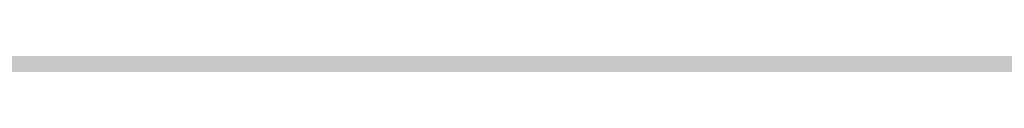
# Model space of a CAD drawing. Units: inches. Extents: x 2091 to 2899, y 967 to 2217.
# Tile 224 of 256: x 2203.4104 to 2203.7172, y 1152.2475 to 1152.2479. Entities that reach past the tile are written whole.
import ezdxf

# ---------------------------------------------------------------- set-up
doc = ezdxf.new("R2010")
doc.units = ezdxf.units.IN
doc.layers.add('A-WALL-PATT', color=141, linetype='Continuous', lineweight=13, true_color=0xadddf7)

msp = doc.modelspace()

# ---------------------------------------------------------------- hatches: boundary and pattern name
at = {"layer": 'A-WALL-PATT'}
h = msp.add_hatch(color=256, dxfattribs=at)
h.dxf.hatch_style = 1
h.paths.add_polyline_path([(2803.1436, 2050.91906), (2203.1436, 2050.91906), (2203.1436, 1090.91906), (2803.1436, 1090.91906)])
h.paths.add_polyline_path([(2635.79885, 1147.54046), (2674.52405, 1147.54046, 0.376086), (2678.52967, 1152.8802), (2678.52967, 1159.55647, 0.333335), (2674.52432, 1163.56185), (2674.52432, 1163.56185), (2674.52432, 1192.93439), (2635.80597, 1192.93439), (2597.08762, 1192.93439), (2597.08762, 1163.56185, 0.333335), (2593.08228, 1159.55647), (2593.08228, 1152.8802, 0.376086), (2597.08789, 1147.54046)], flags=0)
h.paths.add_polyline_path([(2436.01043, 1278.24078, 0.000483), (2435.95264, 1278.21503, -0.001328), (2435.93563, 1278.11169, -0.001711), (2436.11644, 1278.04076, 0.002185)], flags=0)
h.paths.add_polyline_path([(2794.1436, 1143.41906), (2794.1436, 1347.41906), (2543.37017, 1347.41906), (2543.37017, 1351.91906), (2794.1436, 1351.91906), (2794.1436, 1392.71355), (2793.9474, 1392.71355), (2793.9474, 1473.5369), (2794.1436, 1473.5369), (2794.1436, 1531.91906), (2650.1436, 1531.91906), (2650.1436, 1536.41906), (2794.1436, 1536.41906), (2794.1436, 1692.41906), (2609.37561, 1692.41906), (2609.37561, 1644.41906), (2604.87561, 1644.41906), (2604.87561, 1744.91906), (2609.37561, 1744.91906), (2609.37561, 1696.91906), (2794.1436, 1696.91906), (2794.1436, 1780.91906), (2609.6436, 1780.91906), (2493.87561, 1780.91906), (2493.87561, 1785.41906), (2609.6436, 1785.41906), (2794.1436, 1785.41906), (2794.1436, 1847.93882), (2793.95122, 1847.93882), (2793.95122, 1928.76217), (2794.1436, 1928.76217), (2794.1436, 1941.41906), (2614.1436, 1941.41906), (2614.1436, 1821.41906), (2609.6436, 1821.41906), (2609.6436, 1941.41906), (2392.1436, 1941.41906), (2392.1436, 1819.91906), (2387.6436, 1819.91906), (2387.6436, 1941.41906), (2212.1436, 1941.41906), (2212.1436, 1783.91906), (2392.1436, 1783.91906), (2392.1436, 1780.91906), (2212.1436, 1780.91906), (2212.1436, 1629.41906), (2387.6436, 1629.41906), (2387.6436, 1744.91906), (2392.1436, 1744.91906), (2392.1436, 1627.91906), (2317.1436, 1627.91906), (2317.1436, 1551.41906), (2317.1436, 1536.41906), (2459.38359, 1536.41906), (2459.38359, 1602.39648), (2463.88359, 1602.39648), (2463.88359, 1531.91906), (2456.6436, 1531.91906), (2456.6436, 1529.91906), (2452.1436, 1529.91906), (2452.1436, 1531.91906), (2312.6436, 1531.91906), (2312.6436, 1551.41906), (2306.1436, 1551.41906), (2306.1436, 1555.91906), (2308.1436, 1555.91906), (2308.1436, 1551.41906), (2312.6436, 1551.41906), (2312.6436, 1627.91906), (2212.1436, 1627.91906), (2212.1436, 1555.91906), (2270.1436, 1555.91906), (2270.1436, 1551.41906), (2212.1436, 1551.41906), (2212.1436, 1351.91906), (2272.1436, 1351.91906), (2272.1436, 1347.41906), (2212.1436, 1347.41906), (2212.1436, 1275.41906), (2308.1436, 1275.41906), (2308.1436, 1351.91906), (2452.1436, 1351.91906), (2452.1436, 1493.91906), (2456.6436, 1493.91906), (2456.6436, 1347.41906), (2312.6436, 1347.41906), (2312.6436, 1270.91906), (2212.1436, 1270.91906), (2212.1436, 1099.91906), (2281.23752, 1099.91906), (2282.87104, 1110.9138), (2282.00834, 1116.9966), (2278.55774, 1121.4204), (2268.20564, 1128.0562), (2272.08764, 1128.0562), (2273.81294, 1131.927), (2279.42034, 1134.6919), (2285.02784, 1135.2449), (2287.61584, 1137.4568), (2288.04714, 1138.0098), (2289.34114, 1140.7747), (2291.06654, 1139.6687), (2292.36054, 1135.2449), (2295.37984, 1136.9038), (2296.24254, 1135.7979), (2297.10524, 1133.033), (2300.12464, 1138.0098), (2303.14394, 1138.0098), (2304.43794, 1135.7979), (2303.14394, 1133.586), (2306.59464, 1134.6919), (2307.88874, 1133.033), (2310.90804, 1135.2449), (2313.92744, 1134.1389), (2315.62686, 1132.4271), (2308.32004, 1117.5496), (2290.20384, 1109.8079), (2288.90984, 1103.1721), (2289.27231, 1099.91906), (2434.91823, 1099.91906), (2431.59323, 1124.78806), (2429.93023, 1169.55306), (2430.92718, 1240.51969), (2435.65893, 1238.18613), (2437.13523, 1196.55406), (2438.79823, 1143.97306), (2442.67823, 1111.99806), (2446.55823, 1099.91906), (2794.1436, 1099.91906), (2794.1436, 1138.91906), (2548.03245, 1138.91906), (2548.03245, 1143.41906), (2548.03245, 1148.81906), (2546.66846, 1148.03156), (2528.68569, 1179.17862, 0.256256), (2512.03245, 1148.81906), (2512.03245, 1143.41906), (2512.03245, 1138.91906), (2507.53245, 1138.91906), (2507.53245, 1143.41906), (2507.53245, 1148.81906, 0.256256), (2490.8792, 1179.17862), (2472.89644, 1148.03156), (2471.53245, 1148.81906), (2471.53245, 1143.41906), (2467.03245, 1143.41906), (2467.03245, 1269.94579, 0.039061), (2460.90999, 1273.58006), (2467.03245, 1273.58006), (2467.03245, 1286.32536, 0.014511), (2465.21619, 1286.76191), (2467.03245, 1287.05258), (2467.03245, 1323.41906), (2471.53245, 1323.41906), (2471.53245, 1148.81906), (2489.53245, 1179.99597), (2490.89644, 1179.20847), (2490.8792, 1179.17862, -0.256256), (2507.53245, 1148.81906), (2507.53245, 1143.41906), (2512.03245, 1143.41906), (2512.03245, 1148.81906, -0.256256), (2528.68569, 1179.17862), (2528.66846, 1179.20847), (2530.03245, 1179.99597), (2548.03245, 1148.81906), (2548.03245, 1143.41906)], flags=16)
h.paths.add_polyline_path([(2607.76855, 1200.94508), (2607.76855, 1265.03063), (2597.08762, 1281.05201), (2619.78459, 1281.05201), (2627.79528, 1337.12686), (2635.79885, 1337.12686), (2643.81666, 1337.12686), (2651.82736, 1281.05201), (2674.52432, 1281.05201), (2663.8434, 1265.03063), (2663.8434, 1200.94508), (2635.80597, 1200.94508)], flags=0)
edge = h.paths.add_edge_path(flags=0)
edge.add_ellipse((13303.89622, 1272.99872), major_axis=(-10595.31304, 0), ratio=0.84230387009, start_angle=0.628237219, end_angle=0.6465541, ccw=False)
edge.add_ellipse((2711.70045, 1156.85268), major_axis=(2.21977, 0), ratio=0.8423039, start_angle=111.53524, end_angle=180.62824, ccw=False)
edge.add_ellipse((13303.15629, 1272.99872), major_axis=(-10593.02631, 0), ratio=0.84230386954, start_angle=0.528271472, end_angle=0.646554097, ccw=False)
edge.add_line((2710.7646, 1175.3333), (2710.12999, 1175.3333))
edge.add_ellipse((2710.12999, 1176.57978), major_axis=(1.47985, 0), ratio=0.8423039, start_angle=180, end_angle=270, ccw=False)
edge.add_line((2708.65014, 1176.57978), (2708.65014, 1200.78291))
edge.add_ellipse((2710.12999, 1200.78291), major_axis=(1.47985, 0), ratio=0.8423039, start_angle=90, end_angle=180, ccw=False)
edge.add_line((2710.12999, 1202.02939), (2710.46508, 1202.02939))
edge.add_ellipse((13303.15629, 1272.99872), major_axis=(-10593.02631, 0), ratio=0.84230386954, start_angle=-0.090229089, end_angle=0.383866779, ccw=False)
edge.add_ellipse((2710.12999, 1290.92703), major_axis=(-1.47985, 0), ratio=0.8423039, start_angle=0, end_angle=90, ccw=False)
edge.add_line((2708.65014, 1290.92703), (2708.65014, 1315.13017))
edge.add_ellipse((2710.12999, 1315.13017), major_axis=(-1.47985, 0), ratio=0.8423039, start_angle=-90, end_angle=0, ccw=False)
edge.add_line((2710.12999, 1316.37665), (2710.70631, 1316.37665))
edge.add_ellipse((3238.40172, 1296.28957), major_axis=(528.234, 0), ratio=0.84230387, start_angle=176.3495724, end_angle=177.8200497, ccw=False)
edge.add_ellipse((2775.06304, 1071.4507), major_axis=(313.30776, 0), ratio=0.84230387, start_angle=102.1259656, end_angle=103.780529, ccw=False)
edge.add_ellipse((2775.06304, 1078.3057), major_axis=(-305.30289, 0), ratio=0.84230387, start_angle=-79.790461, end_angle=-77.5553727, ccw=False)
edge.add_ellipse((2695.14177, 1541.97538), major_axis=(-250.96022, 0), ratio=0.84230387, start_angle=99.256566, end_angle=102.5549326)
edge.add_line((2741.41033, 1334.21426), (2747.13255, 1337.37848))
edge.add_ellipse((2747.53862, 1336.85748), major_axis=(-0.73992, 0), ratio=0.842304, start_angle=270, end_angle=307.93313, ccw=False)
edge.add_ellipse((2747.53862, 1336.85748), major_axis=(-0.73992, 0), ratio=0.842304, start_angle=232.06687, end_angle=270, ccw=False)
edge.add_line((2747.94469, 1337.37848), (2753.66691, 1334.21426))
edge.add_ellipse((2799.93547, 1541.97538), major_axis=(250.96022, 0), ratio=0.84230387, start_angle=257.4450674, end_angle=260.743434)
edge.add_ellipse((2720.01419, 1078.3057), major_axis=(305.30289, 0), ratio=0.84230387, start_angle=77.5553727, end_angle=79.790461, ccw=False)
edge.add_ellipse((2720.01419, 1071.4507), major_axis=(-313.30776, 0), ratio=0.84230387, start_angle=256.219471, end_angle=257.8740344, ccw=False)
edge.add_ellipse((2256.67551, 1296.28957), major_axis=(-528.234, 0), ratio=0.84230387, start_angle=182.1799503, end_angle=183.6504276, ccw=False)
edge.add_line((2784.37092, 1316.37665), (2784.94725, 1316.37665))
edge.add_ellipse((2784.94725, 1315.13017), major_axis=(1.47985, 0), ratio=0.8423039, start_angle=0, end_angle=90, ccw=False)
edge.add_line((2786.42709, 1315.13017), (2786.42709, 1290.92703))
edge.add_ellipse((2784.94725, 1290.92703), major_axis=(1.47985, 0), ratio=0.8423039, start_angle=270, end_angle=360, ccw=False)
edge.add_ellipse((-7808.07906, 1272.99872), major_axis=(10593.02631, 0), ratio=0.84230386954, start_angle=-0.383866779, end_angle=0.090229089, ccw=False)
edge.add_line((2784.61216, 1202.02939), (2784.94725, 1202.02939))
edge.add_ellipse((2784.94725, 1200.78291), major_axis=(1.47985, 0), ratio=0.8423039, start_angle=0, end_angle=90, ccw=False)
edge.add_line((2786.42709, 1200.78291), (2786.42709, 1176.57978))
edge.add_ellipse((2784.94725, 1176.57978), major_axis=(-1.47985, 0), ratio=0.8423039, start_angle=90, end_angle=180, ccw=False)
edge.add_line((2784.94725, 1175.3333), (2784.31264, 1175.3333))
edge.add_ellipse((-7808.07906, 1272.99872), major_axis=(10593.02631, 0), ratio=0.84230386954, start_angle=-0.618643196, end_angle=-0.528271472, ccw=False)
edge.add_ellipse((2783.37678, 1156.85268), major_axis=(-2.21977, 0), ratio=0.8423039, start_angle=179.37176, end_angle=248.46476, ccw=False)
edge.add_ellipse((-7808.81898, 1272.99872), major_axis=(-10595.31304, 0), ratio=0.84230386576, start_angle=179.353445923, end_angle=179.371762803, ccw=False)
edge.add_ellipse((2780.2973, 1153.50079), major_axis=(-5.24643, 0), ratio=0.8423039, start_angle=90, end_angle=179.35345, ccw=False)
edge.add_line((2780.2973, 1149.08171), (2714.77993, 1149.08171))
edge.add_ellipse((2714.77993, 1153.50079), major_axis=(5.24643, 0), ratio=0.8423039, start_angle=180.64655, end_angle=270, ccw=False)
edge = h.paths.add_edge_path(flags=0)
edge.add_line((2718.18737, 1151.00783), (2718.18737, 1170.47236))
edge.add_ellipse((2721.14706, 1170.47236), major_axis=(-2.95969, 0), ratio=0.8423039, start_angle=-90, end_angle=0, ccw=False)
edge.add_line((2721.14706, 1172.96532), (2773.93017, 1172.96532))
edge.add_ellipse((2773.93017, 1170.47236), major_axis=(-2.95969, 0), ratio=0.8423039, start_angle=180, end_angle=270, ccw=False)
edge.add_line((2776.88987, 1170.47236), (2776.88987, 1151.00783))
edge.add_line((2776.88987, 1151.00783), (2718.18737, 1151.00783))
edge = h.paths.add_edge_path(flags=0)
edge.add_line((2718.18737, 1180.23415), (2718.18737, 1199.05783))
edge.add_ellipse((2747.53862, 1320.39864), major_axis=(147.01792, 0), ratio=0.84230387, start_angle=256.4018653, end_angle=283.5981347)
edge.add_line((2776.88987, 1199.05783), (2776.88987, 1180.23415))
edge.add_ellipse((2747.53862, 1301.57496), major_axis=(147.01792, 0), ratio=0.84230387, start_angle=256.4018653, end_angle=283.5981347, ccw=False)
edge = h.paths.add_edge_path(flags=0)
edge.add_ellipse((13303.15629, 1272.99872), major_axis=(-10591.54646, 0), ratio=0.84230386955, start_angle=0.055594314, end_angle=0.377764194, ccw=False)
edge.add_line((2711.61686, 1262.72171), (2715.66741, 1249.4954))
edge.add_ellipse((6413.89196, 1241.69192), major_axis=(-3698.23616, 0), ratio=0.8423038695, start_angle=-0.12089737, end_angle=0.36407635)
edge.add_line((2715.76104, 1218.19245), (2711.93431, 1203.16736))
edge = h.paths.add_edge_path(flags=0)
edge.add_line((2718.18737, 1251.07457), (2716.00249, 1267.45044))
edge.add_ellipse((2742.15117, 1202.18954), major_axis=(81.77258, 0), ratio=0.84230387, start_angle=94.277421, end_angle=111.8349538, ccw=False)
edge.add_line((2737.00975, 1270.93063), (2758.06748, 1270.93063))
edge.add_ellipse((2752.92606, 1202.18954), major_axis=(81.77258, 0), ratio=0.84230387, start_angle=68.1650462, end_angle=85.722579, ccw=False)
edge.add_line((2779.07475, 1267.45044), (2776.88987, 1251.07457))
edge.add_ellipse((2750.33806, 1187.88536), major_axis=(79.57966, 0), ratio=0.84230387, start_angle=67.2080851, end_angle=85.1299304)
edge.add_line((2756.03466, 1254.74366), (2739.04258, 1254.74366))
edge.add_ellipse((2744.73917, 1187.88536), major_axis=(79.57966, 0), ratio=0.84230387, start_angle=94.8700696, end_angle=112.7919149)
edge = h.paths.add_edge_path(flags=0)
edge.add_line((2783.14293, 1203.16736), (2779.31619, 1218.19245))
edge.add_ellipse((-918.81473, 1241.69192), major_axis=(3698.23616, 0), ratio=0.8423038695, start_angle=-0.36407635, end_angle=0.12089737)
edge.add_line((2779.40983, 1249.4954), (2783.46037, 1262.72171))
edge.add_ellipse((-7808.07906, 1272.99872), major_axis=(-10591.54646, 0), ratio=0.84230386954, start_angle=179.622235806, end_angle=179.944405687, ccw=False)
edge = h.paths.add_edge_path(flags=0)
edge.add_ellipse((2734.20089, 1286.69044), major_axis=(-0.35661, 6.34008), ratio=0.6038336, start_angle=89.002014, end_angle=253.657408, ccw=False)
edge.add_line((2730.369, 1286.54181), (2730.369, 1301.35198))
edge.add_line((2730.369, 1301.35198), (2735.91331, 1305.2148))
edge.add_ellipse((2736.38492, 1304.73456), major_axis=(0.73992, 0), ratio=0.842304, start_angle=90, end_angle=134.48021, ccw=False)
edge.add_line((2736.38492, 1305.3578), (2738.03278, 1305.3578))
edge.add_line((2738.03278, 1305.3578), (2738.03278, 1307.70793))
edge.add_ellipse((2794.20164, 1307.70793), major_axis=(56.16886, 0), ratio=0.84230387, start_angle=150.56143, end_angle=180, ccw=False)
edge.add_ellipse((2700.87559, 1307.70793), major_axis=(-56.16886, 0), ratio=0.84230387, start_angle=180, end_angle=209.43857, ccw=False)
edge.add_line((2757.04445, 1307.70793), (2757.04445, 1305.3578))
edge.add_line((2757.04445, 1305.3578), (2758.69232, 1305.3578))
edge.add_ellipse((2758.69232, 1304.73456), major_axis=(-0.73992, 0), ratio=0.842304, start_angle=225.51979, end_angle=270, ccw=False)
edge.add_line((2759.16392, 1305.2148), (2764.70823, 1301.35198))
edge.add_line((2764.70823, 1301.35198), (2764.70823, 1286.54181))
edge.add_ellipse((2760.87634, 1286.69044), major_axis=(0.35661, 6.34008), ratio=0.6038336, start_angle=106.342592, end_angle=270.997986, ccw=False)
edge.add_line((2757.04445, 1285.79709), (2757.04445, 1307.70793))
edge.add_ellipse((2700.87559, 1307.70793), major_axis=(-56.16886, 0), ratio=0.84230387, start_angle=180, end_angle=209.43857)
edge.add_ellipse((2794.20164, 1307.70793), major_axis=(56.16886, 0), ratio=0.84230387, start_angle=150.56143, end_angle=180)
edge.add_line((2738.03278, 1307.70793), (2738.03278, 1285.79709))
h.paths.add_polyline_path([(2417.81227, 1104.4497), (2413.49227, 1102.5297), (2410.61227, 1103.9697), (2409.17227, 1106.3697), (2407.25227, 1107.3297), (2406.29227, 1109.7297), (2405.33227, 1114.0497), (2405.33227, 1117.8897), (2406.29227, 1120.1297), (2407.25227, 1119.8097), (2408.84832, 1118.32766), (2410.17395, 1119.42417), (2410.21127, 1120.4057), (2411.04073, 1121.41905), (2410.69927, 1119.8587), (2410.17395, 1119.42417), (2410.08845, 1117.17611), (2411.13284, 1116.20632), (2413.97227, 1119.3297), (2416.85227, 1120.7697), (2416.86972, 1120.79878), (2417.03507, 1119.40512), (2417.89621, 1118.14338), (2418.29227, 1118.3697), (2419.54445, 1120.03927), (2419.36092, 1118.38749), (2419.03211, 1119.35615), (2418.39894, 1118.51193), (2419.25227, 1114.5297), (2418.79409, 1107.19879)], flags=0)
h.paths.add_polyline_path([(2508.87017, 1347.41906), (2508.37017, 1347.41906), (2508.37017, 1351.91906), (2508.87017, 1351.91906)], flags=0)
h.paths.add_polyline_path([(2473.37017, 1347.41906), (2472.37017, 1347.41906), (2467.87017, 1347.41906), (2467.87017, 1455.41906), (2472.37017, 1455.41906), (2472.37017, 1352.41906), (2473.37017, 1352.41906)], flags=0)
h.paths.add_polyline_path([(2352.10624, 1217.4462), (2349.22624, 1218.8862), (2347.78624, 1221.2862), (2345.86624, 1222.2462), (2344.90624, 1224.6462), (2343.94624, 1228.9662), (2343.94624, 1232.8062), (2344.90624, 1235.0462), (2345.86624, 1234.7262), (2347.46229, 1233.24415), (2348.78792, 1234.34066), (2348.82524, 1235.3222), (2349.6547, 1236.33555), (2349.31324, 1234.7752), (2348.78792, 1234.34066), (2348.70242, 1232.0926), (2349.74681, 1231.12282), (2352.58624, 1234.2462), (2355.46624, 1235.6862), (2355.48369, 1235.71528), (2355.64904, 1234.32161), (2356.51018, 1233.05988), (2356.90624, 1233.2862), (2358.15842, 1234.95576), (2357.97489, 1233.30398), (2357.64608, 1234.27264), (2357.01291, 1233.42842), (2357.86624, 1229.4462), (2357.40806, 1222.11529), (2356.42624, 1219.3662)], flags=0)
h.paths.add_polyline_path([(2348.2968, 1112.22442), (2347.0138, 1112.31042), (2345.5298, 1114.12742), (2345.7318, 1115.85842), (2346.8118, 1116.98242), (2346.8118, 1114.64642), (2345.8668, 1114.21442), (2346.8798, 1114.30042)], flags=0)
h.paths.add_polyline_path([(2347.0138, 1110.92642), (2346.2718, 1110.49342), (2346.6098, 1111.18642)], flags=0)
h.paths.add_polyline_path([(2345.8668, 1118.19442), (2345.5298, 1117.32942), (2343.7078, 1118.02142), (2344.3828, 1118.62642)], flags=0)
h.paths.add_polyline_path([(2346.6768, 1109.28242), (2346.0698, 1108.07142), (2345.8668, 1110.06142)], flags=0)
h.paths.add_polyline_path([(2345.0568, 1119.75142), (2343.6398, 1119.75142), (2343.9778, 1121.13542)], flags=0)
h.paths.add_polyline_path([(2345.2598, 1116.55042), (2345.1248, 1115.85842), (2344.9218, 1115.68542), (2344.7198, 1116.37742)], flags=0)
h.paths.add_polyline_path([(2345.6648, 1112.31042), (2345.4618, 1111.53242), (2344.0448, 1111.96442), (2344.6518, 1112.57042)], flags=0)
h.paths.add_polyline_path([(2345.1918, 1113.34942), (2344.4498, 1113.86842), (2344.7198, 1114.38742)], flags=0)
h.paths.add_polyline_path([(2344.6518, 1116.80942), (2344.1798, 1115.68542), (2344.6518, 1115.33942), (2343.9098, 1114.90642), (2343.0328, 1115.94442), (2343.6398, 1116.46342)], flags=0)
h.paths.add_polyline_path([(2345.8668, 1106.68642), (2344.9898, 1105.56242), (2344.5168, 1106.60042)], flags=0)
h.paths.add_polyline_path([(2344.8548, 1110.06142), (2344.5168, 1109.28242), (2344.1128, 1109.71542)], flags=0)
h.paths.add_polyline_path([(2344.0448, 1113.52242), (2343.4378, 1113.08942), (2342.7628, 1113.95442)], flags=0)
h.paths.add_polyline_path([(2344.3148, 1111.01242), (2342.9648, 1110.32042), (2342.9648, 1111.09942)], flags=0)
h.paths.add_polyline_path([(2345.1248, 1104.69742), (2344.5848, 1103.74542), (2344.4498, 1104.26442)], flags=0)
h.paths.add_polyline_path([(2342.8298, 1121.22242), (2341.7498, 1120.53042), (2340.5358, 1121.04942), (2340.1308, 1121.82842), (2340.6708, 1122.95242), (2341.1428, 1121.82842), (2341.6148, 1122.00142)], flags=0)
h.paths.add_polyline_path([(2342.9648, 1119.75142), (2343.0328, 1118.45342), (2342.0878, 1118.02142), (2342.0198, 1119.49142)], flags=0)
h.paths.add_polyline_path([(2342.6948, 1116.89642), (2341.9528, 1116.63642), (2342.0198, 1117.32942)], flags=0)
h.paths.add_polyline_path([(2343.0328, 1112.22442), (2342.0198, 1111.79142), (2341.5478, 1112.22442), (2342.3578, 1113.34942)], flags=0)
h.paths.add_polyline_path([(2343.7748, 1104.43742), (2342.6278, 1102.88042), (2342.6948, 1104.61042), (2343.4378, 1105.12942)], flags=0)
h.paths.add_polyline_path([(2342.0198, 1115.07942), (2340.8058, 1115.51242), (2340.9408, 1116.37742)], flags=0)
h.paths.add_polyline_path([(2341.4808, 1120.09742), (2341.4808, 1119.40542), (2341.0758, 1119.57842), (2341.1428, 1120.09742)], flags=0)
h.paths.add_polyline_path([(2341.8178, 1114.47342), (2340.9408, 1113.08942), (2340.8058, 1114.56042)], flags=0)
h.paths.add_polyline_path([(2341.1428, 1118.54042), (2340.9408, 1116.98242), (2339.0508, 1117.67542), (2339.0508, 1118.62642)], flags=0)
h.paths.add_polyline_path([(2342.6948, 1101.66842), (2341.9528, 1101.84142), (2342.5598, 1102.36142)], flags=0)
h.paths.add_polyline_path([(2340.3328, 1119.66542), (2338.4438, 1119.57842), (2337.9038, 1120.35742), (2339.6578, 1120.61642)], flags=0)
h.paths.add_polyline_path([(2340.3328, 1115.33942), (2340.0628, 1113.69542), (2339.3878, 1115.33942)], flags=0)
h.paths.add_polyline_path([(2341.8178, 1103.83142), (2341.5478, 1102.88042), (2341.1428, 1103.65842)], flags=0)
h.paths.add_polyline_path([(2339.0508, 1122.86642), (2337.2958, 1121.82842), (2337.0938, 1123.12542), (2337.7688, 1123.81842)], flags=0)
h.paths.add_polyline_path([(2339.1178, 1121.74142), (2338.8478, 1121.22242), (2338.1738, 1121.04942), (2338.3758, 1121.56842)], flags=0)
h.paths.add_polyline_path([(2339.1858, 1119.31942), (2338.6458, 1118.71342), (2338.2408, 1118.10742), (2338.2408, 1118.88642)], flags=0)
h.paths.add_polyline_path([(2341.1428, 1101.92842), (2340.6028, 1101.23642), (2340.0628, 1101.84142), (2340.6028, 1102.36142)], flags=0)
h.paths.add_polyline_path([(2337.6338, 1117.76142), (2336.6208, 1118.28042), (2337.2958, 1118.97242)], flags=0)
h.paths.add_polyline_path([(2336.8238, 1119.57842), (2334.7988, 1118.97242), (2335.2038, 1120.35742), (2336.5538, 1120.87642)], flags=0)
h.paths.add_polyline_path([(2339.1178, 1100.45742), (2337.3638, 1100.54342), (2336.7558, 1101.23642)], flags=0)
h.paths.add_polyline_path([(2336.3508, 1122.43342), (2336.0138, 1121.91442), (2334.9338, 1122.43342), (2334.5288, 1123.47142), (2335.7438, 1122.77942)], flags=0)
h.paths.add_polyline_path([(2334.7318, 1120.87642), (2334.2588, 1120.35742), (2334.0568, 1120.78942), (2334.5968, 1121.30842)], flags=0)
h.paths.add_polyline_path([(2334.4618, 1122.17442), (2332.5718, 1121.30842), (2331.3568, 1122.17442), (2332.0998, 1122.86642)], flags=0)
h.paths.add_polyline_path([(2334.2588, 1118.54042), (2333.3818, 1118.45342), (2333.6518, 1119.31942)], flags=0)
h.paths.add_polyline_path([(2335.5418, 1102.27442), (2334.1918, 1102.62042), (2335.2718, 1103.31242)], flags=0)
h.paths.add_polyline_path([(2332.7068, 1119.66542), (2331.6948, 1120.44342), (2332.5048, 1120.78942)], flags=0)
h.paths.add_polyline_path([(2334.7318, 1101.14942), (2333.5168, 1101.58242), (2333.9888, 1101.75542)], flags=0)
h.paths.add_polyline_path([(2332.6398, 1116.63642), (2331.0868, 1116.29042), (2331.9648, 1118.19442)], flags=0)
h.paths.add_polyline_path([(2330.7498, 1121.56842), (2330.2768, 1120.27042), (2328.5228, 1119.31942), (2328.9948, 1121.04942)], flags=0)
h.paths.add_polyline_path([(2330.7498, 1118.62642), (2330.0078, 1117.50242), (2329.8728, 1118.02142)], flags=0)
h.paths.add_polyline_path([(2332.0998, 1102.36142), (2330.5468, 1102.01442), (2331.6948, 1102.96642)], flags=0)
h.paths.add_polyline_path([(2329.5348, 1113.60842), (2329.0628, 1112.31042), (2328.5898, 1113.34942)], flags=0)
h.paths.add_polyline_path([(2328.3878, 1117.84842), (2327.5098, 1116.55042), (2327.1728, 1117.76142)], flags=0)
h.paths.add_polyline_path([(2329.7378, 1106.51342), (2329.5348, 1105.30242), (2328.2528, 1106.08142)], flags=0)
h.paths.add_polyline_path([(2328.6578, 1114.38742), (2328.0498, 1114.12742), (2328.3198, 1114.90642)], flags=0)
h.paths.add_polyline_path([(2328.3198, 1112.22442), (2327.1058, 1112.13742), (2326.7008, 1112.65642)], flags=0)
h.paths.add_polyline_path([(2326.9028, 1115.25242), (2326.7008, 1114.12742), (2325.2158, 1113.60842), (2326.0928, 1115.33942)], flags=0)
h.paths.add_polyline_path([(2326.6328, 1108.33042), (2326.0928, 1107.37942), (2325.8908, 1108.50342), (2326.4978, 1109.10942)], flags=0)
h.paths.add_polyline_path([(2615.1436, 1531.91906), (2609.6436, 1531.91906), (2609.6436, 1620.41906), (2614.1436, 1620.41906), (2614.1436, 1536.41906), (2615.1436, 1536.41906)], flags=0)
h.paths.add_polyline_path([(2545.1436, 1563.41906), (2464.1436, 1563.41906), (2464.1436, 1632.41906), (2509.1436, 1632.41906), (2509.1436, 1627.91906), (2509.1436, 1603.91906), (2468.6436, 1603.91906), (2468.6436, 1567.91906), (2540.6436, 1567.91906), (2540.6436, 1591.91906), (2545.1436, 1591.91906)], flags=0)
h.paths.add_polyline_path([(2388.96905, 1549.98573), (2357.43418, 1549.98573), (2357.43418, 1623.36078), (2399.36278, 1623.36078), (2435.68947, 1623.36078), (2435.59255, 1602.55927), (2435.59255, 1602.39648), (2388.96905, 1602.39648)], flags=0)
h.paths.add_polyline_path([(2388.88063, 1555.80915), (2374.90443, 1555.80915), (2374.90443, 1600.57156), (2374.90443, 1615.45765), (2406.35088, 1615.45765), (2406.35088, 1618.93943), (2412.17429, 1615.45765), (2406.35088, 1611.97586), (2406.35088, 1615.45765), (2388.88063, 1615.45765)], flags=0)
h.paths.add_polyline_path([(2568.87561, 1644.41906), (2453.37561, 1644.41906), (2453.37561, 1785.41906), (2457.87561, 1785.41906), (2457.87561, 1648.91906), (2568.87561, 1648.91906)], flags=0)
h.paths.add_polyline_path([(2212.1436, 1945.91906), (2212.1436, 2041.91906), (2794.1436, 2041.91906), (2794.1436, 1945.91906)], flags=16)
h.paths.add_polyline_path([(2271.08273, 1964.31724), (2776.85297, 1964.31724), (2776.85297, 2037.16962), (2271.08273, 2037.16962)], flags=8)
h.paths.add_polyline_path([(2380.64929, 1536.82414), (2461.04081, 1536.82414), (2461.04081, 1554.65259), (2380.64929, 1554.65259)], flags=8)
h.paths.add_polyline_path([(2240.75571, 1609.72545), (2309.18583, 1609.72545), (2309.18583, 1617.6982), (2240.75571, 1617.6982)], flags=8)
h.paths.add_polyline_path([(2212.67726, 1313.5041), (2282.59152, 1313.5041), (2282.59152, 1322.74524), (2212.67726, 1322.74524)], flags=8)
h.paths.add_polyline_path([(2457.11198, 1114.77857), (2558.48158, 1114.77857), (2558.48158, 1142.21968), (2457.11198, 1142.21968)], flags=8)
h.paths.add_polyline_path([(2473.44234, 1273.01007), (2604.64123, 1273.01007), (2604.64123, 1318.34693), (2473.44234, 1318.34693)], flags=8)
h.paths.add_polyline_path([(2638.8763, 1626.97743), (2684.25037, 1627.97674), (2684.03848, 1637.59749), (2638.66442, 1636.59819)], flags=8)
h.paths.add_polyline_path([(2537.59055, 1453.79345), (2628.38955, 1453.79345), (2628.38955, 1475.34481), (2537.59055, 1475.34481)], flags=8)
h.paths.add_polyline_path([(2504.13764, 1714.6324), (2554.64719, 1714.6324), (2554.64719, 1730.23771), (2504.13764, 1730.23771)], flags=8)
h.paths.add_polyline_path([(2487.50118, 1575.65187), (2535.09712, 1575.65187), (2535.09712, 1598.37765), (2487.50118, 1598.37765)], flags=8)
h.paths.add_polyline_path([(2709.0994, 1735.71028), (2740.0166, 1735.71028), (2740.0166, 1749.93764), (2709.0994, 1749.93764)], flags=8)
h.paths.add_polyline_path([(2442.43842, 1792.17166), (2564.72884, 1792.17166), (2564.72884, 1842.00016), (2442.43842, 1842.00016)], flags=8)
h.paths.add_polyline_path([(2655.8158, 1809.64408), (2789.52014, 1806.6938), (2790.08498, 1832.29164), (2656.38064, 1835.24192)], flags=8)
h.paths.add_polyline_path([(2234.8427, 1797.72014), (2368.59285, 1794.76885), (2369.16072, 1820.50413), (2235.41056, 1823.45542)], flags=8)
h.paths.add_polyline_path([(2245.13847, 1644.00633), (2398.42773, 1640.6239), (2398.99484, 1666.32482), (2245.70557, 1669.70725)], flags=8)
h.paths.add_polyline_path([(2306.14285, 1431.16852), (2413.76831, 1428.79369), (2414.33315, 1454.39153), (2306.70768, 1456.76636)], flags=8)
h.paths.add_polyline_path([(2306.83458, 1458.23314), (2393.38048, 1456.32345), (2393.93281, 1481.35436), (2307.38691, 1483.26405)], flags=8)

doc.saveas('drawing.dxf')
